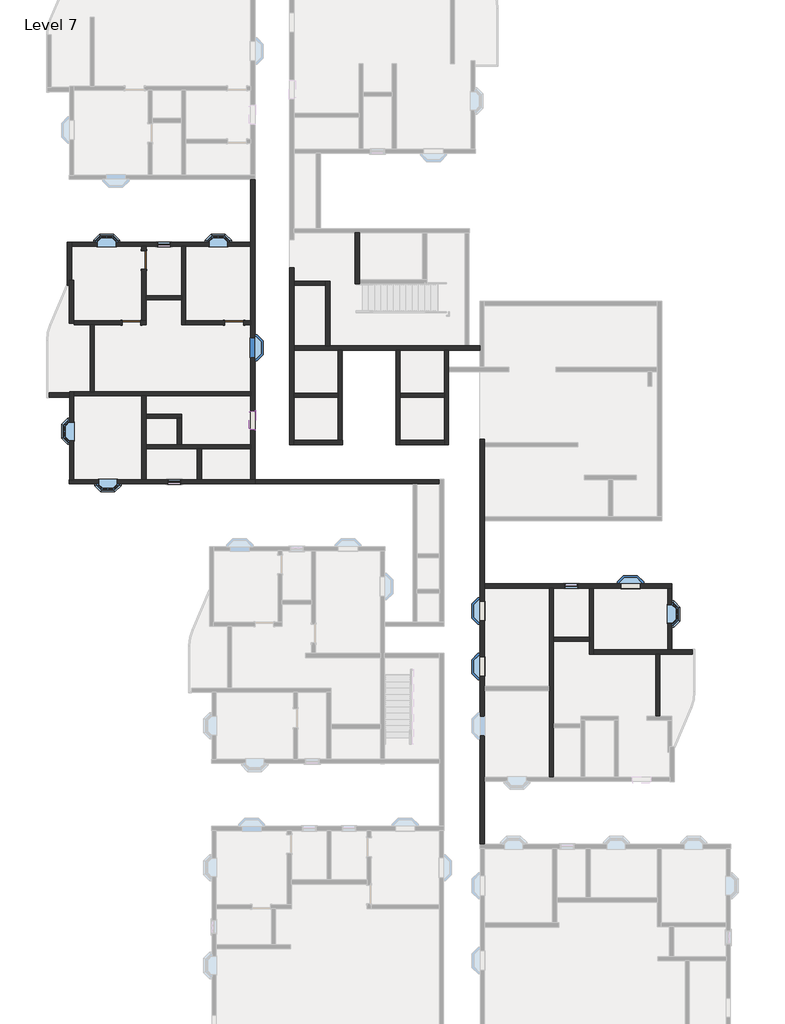
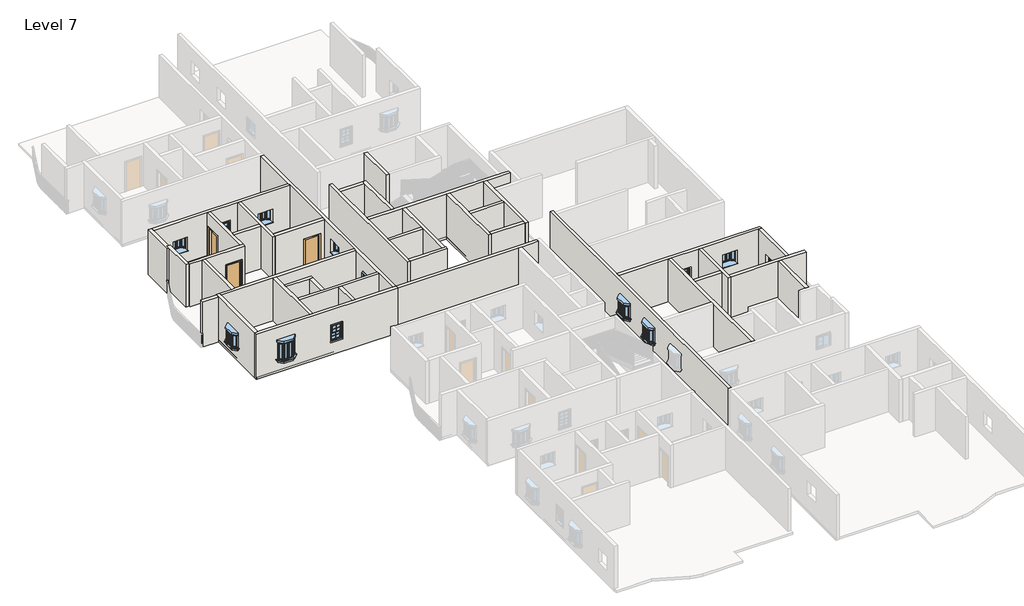
# One storey, part 3 of 14: 40 walls, 13 windows, 3 doors.
"""IFC4 building model written with IfcOpenShell, lengths in millimetres."""

from ifc_helpers import new_model, si_unit, frame, origin, place, context, project, spatial, polyline, outline, extrude, faceted_brep, transform, mapped, element, save
from components import door_54dd4da4, window_910x1210mm_154f9356, window_910x910mm_67ef725a, window_8debb0fa, windows_sgl_w_glazing_bars_910x910mm_256712d0

model = new_model("IFC4")

# Units and contexts
model_context = context("Model", 3, world=origin())
ifc_project = project(units=[si_unit("LENGTHUNIT", "METRE", prefix="MILLI")], contexts=[model_context])

# Site, building, storey
site = spatial("IfcSite", under=ifc_project)
building = spatial("IfcBuilding", under=site)
storey = spatial("IfcBuildingStorey", under=building, Name="Level 7", Elevation=18288.0)

# Doors
placement = place(None, origin())
door_shape = door_54dd4da4(model_context)
element("IfcDoor", 1, ObjectType="Single-Flush : 36\" x 84\"", at=placement, inside=storey, context=model_context, shape_type="MappedRepresentation", body=[
    mapped(door_shape, transform((-11210.3891351, 10605.7083494, 18288.0), x_axis=(1.0, 0.0, 0.0), y_axis=(0.0, 1.0, 0.0), z_axis=(0.0, 0.0, 1.0))),
])
element("IfcDoor", 2, ObjectType="Single-Flush : 36\" x 84\"", at=placement, inside=storey, context=model_context, shape_type="MappedRepresentation", body=[
    mapped(door_shape, transform((-15610.9391351, 13672.7583494, 18288.0), x_axis=(0.0, -1.0, 0.0), y_axis=(1.0, 0.0, 0.0), z_axis=(0.0, 0.0, 1.0))),
])
element("IfcDoor", 3, ObjectType="Single-Flush : 36\" x 84\"", at=placement, inside=storey, context=model_context, shape_type="MappedRepresentation", body=[
    mapped(door_shape, transform((-16220.5391351, 10605.7083494, 18288.0), x_axis=(1.0, 0.0, 0.0), y_axis=(0.0, 1.0, 0.0), z_axis=(0.0, 0.0, 1.0))),
])

# Walls
element("IfcWall", 4, ObjectType="4.5\" p", at=placement, inside=storey, context=model_context, shape_type="Brep", body=[
    faceted_brep([(-15509.3391351, 4456.3873146, 18288.0), (-13007.4391351, 4456.3873146, 18288.0), (-12804.2391351, 4456.3873146, 18288.0), (-10397.5891351, 4456.3873146, 18288.0), (-10397.5891351, 4456.3873146, 21336.0), (-12804.2391351, 4456.3873146, 21336.0), (-13007.4391351, 4456.3873146, 21336.0), (-15509.3391351, 4456.3873146, 21336.0), (-15509.3391351, 4659.5873146, 18288.0), (-15509.3391351, 4659.5873146, 21336.0), (-13985.3391351, 4659.5873146, 21336.0), (-13782.1391351, 4659.5873146, 21336.0), (-10397.5891351, 4659.5873146, 21336.0), (-10397.5891351, 4659.5873146, 18288.0), (-13782.1391351, 4659.5873146, 18288.0), (-13985.3391351, 4659.5873146, 18288.0)], [[[0, 1, 2, 3, 4, 5, 6, 7]], [[8, 9, 10, 11, 12, 13, 14, 15]], [[3, 2, 1, 0, 8, 15, 14, 13]], [[7, 6, 5, 4, 12, 11, 10, 9]], [[4, 3, 13, 12]], [[0, 7, 9, 8]]]),
])
element("IfcWall", 5, ObjectType="4.5\" p", at=placement, inside=storey, context=model_context, shape_type="SweptSolid", body=[
    extrude(outline(polyline([(-13007.4391351, 2953.9583494), (-13007.4391351, 4456.3873146), (-12804.2391351, 4456.3873146), (-12804.2391351, 2953.9583494), (-13007.4391351, 2953.9583494)])), frame((0.0, 0.0, 18288.0), z_axis=(0.0, 0.0, 1.0), x_axis=(1.0, 0.0, 0.0)), (0.0, 0.0, 1.0), 3048.0),
])
element("IfcWall", 6, ObjectType="4.5\" p", at=placement, inside=storey, context=model_context, shape_type="Brep", body=[
    faceted_brep([(-15509.3391351, 5953.2975261, 18288.0), (-13985.3391351, 5953.2975261, 18288.0), (-13782.1391351, 5953.2975261, 18288.0), (-13782.1391351, 5953.2975261, 21336.0), (-13985.3391351, 5953.2975261, 21336.0), (-15509.3391351, 5953.2975261, 21336.0), (-15509.3391351, 6156.4975261, 18288.0), (-15509.3391351, 6156.4975261, 21336.0), (-13782.1391351, 6156.4975261, 21336.0), (-13782.1391351, 6156.4975261, 18288.0)], [[[0, 1, 2, 3, 4, 5]], [[6, 7, 8, 9]], [[2, 1, 0, 6, 9]], [[5, 4, 3, 8, 7]], [[0, 5, 7, 6]], [[3, 2, 9, 8]]]),
])
element("IfcWall", 7, ObjectType="4.5\" p", at=placement, inside=storey, context=model_context, shape_type="SweptSolid", body=[
    extrude(outline(polyline([(-13985.3391351, 4659.5873146), (-13985.3391351, 5953.2975261), (-13782.1391351, 5953.2975261), (-13782.1391351, 4659.5873146), (-13985.3391351, 4659.5873146)])), frame((0.0, 0.0, 18288.0), z_axis=(0.0, 0.0, 1.0), x_axis=(1.0, 0.0, 0.0)), (0.0, 0.0, 1.0), 3048.0),
])
element("IfcWall", 8, ObjectType="4.5\" p", at=placement, inside=storey, context=model_context, shape_type="Brep", body=[
    faceted_brep([(-15712.5391351, 13215.5583494, 20421.6), (-15712.5391351, 13215.5583494, 18288.0), (-15712.5391351, 10707.3083494, 18288.0), (-15712.5391351, 10707.3083494, 21336.0), (-15712.5391351, 14333.1583494, 21336.0), (-15712.5391351, 14333.1583494, 18288.0), (-15712.5391351, 14129.9583494, 18288.0), (-15712.5391351, 14129.9583494, 20421.6), (-15509.3391351, 10707.3083494, 18288.0), (-15509.3391351, 11723.3083494, 18288.0), (-15509.3391351, 11926.5083494, 18288.0), (-15509.3391351, 13215.5583494, 18288.0), (-15509.3391351, 13215.5583494, 20421.6), (-15509.3391351, 14129.9583494, 20421.6), (-15509.3391351, 14129.9583494, 18288.0), (-15509.3391351, 14333.1583494, 18288.0), (-15509.3391351, 14333.1583494, 21336.0), (-15509.3391351, 11926.5083494, 21336.0), (-15509.3391351, 11723.3083494, 21336.0), (-15509.3391351, 10707.3083494, 21336.0)], [[[0, 1, 2, 3, 4, 5, 6, 7]], [[8, 9, 10, 11, 12, 13, 14, 15, 16, 17, 18, 19]], [[6, 5, 15, 14]], [[2, 1, 11, 10, 9, 8]], [[4, 3, 19, 18, 17, 16]], [[3, 2, 8, 19]], [[5, 4, 16, 15]], [[12, 11, 1, 0]], [[13, 12, 0, 7]], [[14, 13, 7, 6]]]),
])
element("IfcWall", 9, ObjectType="4.5\" p", at=placement, inside=storey, context=model_context, shape_type="Brep", body=[
    faceted_brep([(-13769.4391351, 14333.1583494, 18288.0), (-13769.4391351, 11926.5083494, 18288.0), (-13769.4391351, 11723.3083494, 18288.0), (-13769.4391351, 10504.1083494, 18288.0), (-13769.4391351, 10504.1083494, 21336.0), (-13769.4391351, 11723.3083494, 21336.0), (-13769.4391351, 11926.5083494, 21336.0), (-13769.4391351, 14333.1583494, 21336.0), (-13566.2391351, 14333.1583494, 18288.0), (-13566.2391351, 14333.1583494, 21336.0), (-13566.2391351, 10707.3083494, 21336.0), (-13566.2391351, 10504.1083494, 21336.0), (-13566.2391351, 10504.1083494, 18288.0), (-13566.2391351, 10707.3083494, 18288.0)], [[[0, 1, 2, 3, 4, 5, 6, 7]], [[8, 9, 10, 11, 12, 13]], [[3, 2, 1, 0, 8, 13, 12]], [[7, 6, 5, 4, 11, 10, 9]], [[0, 7, 9, 8]], [[4, 3, 12, 11]]]),
])
element("IfcWall", 10, ObjectType="4.5\" p", at=placement, inside=storey, context=model_context, shape_type="SweptSolid", body=[
    extrude(outline(polyline([(20421.6, -10753.1891351), (18288.0, -10753.1891351), (18288.0, -10397.5891351), (21336.0, -10397.5891351), (21336.0, -13566.2391351), (18288.0, -13566.2391351), (18288.0, -11667.5891351), (20421.6, -11667.5891351), (20421.6, -10753.1891351)])), frame((0.0, 10504.1083494, 0.0), z_axis=(0.0, 1.0, 0.0), x_axis=(0.0, 0.0, 1.0)), (0.0, 0.0, 1.0), 203.2),
])
element("IfcWall", 11, ObjectType="4.5\" p", at=placement, inside=storey, context=model_context, shape_type="SweptSolid", body=[
    extrude(outline(polyline([(-13769.4391351, 11723.3083494), (-15509.3391351, 11723.3083494), (-15509.3391351, 11926.5083494), (-13769.4391351, 11926.5083494), (-13769.4391351, 11723.3083494)])), frame((0.0, 0.0, 18288.0), z_axis=(0.0, 0.0, 1.0), x_axis=(1.0, 0.0, 0.0)), (0.0, 0.0, 1.0), 3048.0),
])
element("IfcWall", 12, ObjectType="4.5\" p", at=placement, inside=storey, context=model_context, shape_type="SweptSolid", body=[
    extrude(outline(polyline([(-6739.9891351, 12429.8715905), (-8289.3891351, 12429.8715905), (-8289.3891351, 12633.0715905), (-6739.9891351, 12633.0715905), (-6739.9891351, 12429.8715905)])), frame((0.0, 0.0, 18288.0), z_axis=(0.0, 0.0, 1.0), x_axis=(1.0, 0.0, 0.0)), (0.0, 0.0, 1.0), 3048.0),
])
element("IfcWall", 13, ObjectType="4.5\" p", at=placement, inside=storey, context=model_context, shape_type="SweptSolid", body=[
    extrude(outline(polyline([(-6130.3891351, 6970.2449943), (-8289.3891351, 6970.2449943), (-8289.3891351, 7173.4449943), (-6130.3891351, 7173.4449943), (-6130.3891351, 6970.2449943)])), frame((0.0, 0.0, 18288.0), z_axis=(0.0, 0.0, 1.0), x_axis=(1.0, 0.0, 0.0)), (0.0, 0.0, 1.0), 3048.0),
])
element("IfcWall", 14, ObjectType="4.5\" p", at=placement, inside=storey, context=model_context, shape_type="SweptSolid", body=[
    extrude(outline(polyline([(-948.7891351, 6970.2449943), (-3107.7891351, 6970.2449943), (-3107.7891351, 7173.4449943), (-948.7891351, 7173.4449943), (-948.7891351, 6970.2449943)])), frame((0.0, 0.0, 18288.0), z_axis=(0.0, 0.0, 1.0), x_axis=(1.0, 0.0, 0.0)), (0.0, 0.0, 1.0), 3048.0),
])
element("IfcWall", 15, ObjectType="4.5\" p", at=placement, inside=storey, context=model_context, shape_type="Brep", body=[
    faceted_brep([(-5298.5391351, 14988.9215905, 18288.0), (-5298.5391351, 12506.0715905, 18288.0), (-5298.5391351, 12506.0715905, 21336.0), (-5298.5391351, 14988.9215905, 21336.0), (-5095.3391351, 14988.9215905, 18288.0), (-5095.3391351, 14988.9215905, 21336.0), (-5095.3391351, 12709.2715905, 21336.0), (-5095.3391351, 12506.0715905, 21336.0), (-5095.3391351, 12506.0715905, 18288.0), (-5095.3391351, 12709.2715905, 18288.0)], [[[0, 1, 2, 3]], [[4, 5, 6, 7, 8, 9]], [[1, 0, 4, 9, 8]], [[3, 2, 7, 6, 5]], [[0, 3, 5, 4]], [[2, 1, 8, 7]]]),
])
element("IfcWall", 16, ObjectType="4.5\" p", at=placement, inside=storey, context=model_context, shape_type="SweptSolid", body=[
    extrude(outline(polyline([(-948.7891351, 4665.1949943), (-3107.7891351, 4665.1949943), (-3107.7891351, 4868.3949943), (-948.7891351, 4868.3949943), (-948.7891351, 4665.1949943)])), frame((0.0, 0.0, 18288.0), z_axis=(0.0, 0.0, 1.0), x_axis=(1.0, 0.0, 0.0)), (0.0, 0.0, 1.0), 3048.0),
])
element("IfcWall", 17, ObjectType="4.5\" p", at=placement, inside=storey, context=model_context, shape_type="Brep", body=[
    faceted_brep([(4184.4880523, -2336.4042694, 18288.0), (4184.4880523, -7130.6542694, 18288.0), (4184.4880523, -7333.8542694, 18288.0), (4184.4880523, -11556.6042694, 18288.0), (4184.4880523, -11556.6042694, 21336.0), (4184.4880523, -7333.8542694, 21336.0), (4184.4880523, -7130.6542694, 21336.0), (4184.4880523, -2336.4042694, 21336.0), (4387.6880523, -2336.4042694, 18288.0), (4387.6880523, -2336.4042694, 21336.0), (4387.6880523, -4736.7042694, 21336.0), (4387.6880523, -4939.9042694, 21336.0), (4387.6880523, -8959.4542694, 21336.0), (4387.6880523, -9162.6542694, 21336.0), (4387.6880523, -11556.6042694, 21336.0), (4387.6880523, -11556.6042694, 18288.0), (4387.6880523, -9162.6542694, 18288.0), (4387.6880523, -8959.4542694, 18288.0), (4387.6880523, -4939.9042694, 18288.0), (4387.6880523, -4736.7042694, 18288.0)], [[[0, 1, 2, 3, 4, 5, 6, 7]], [[8, 9, 10, 11, 12, 13, 14, 15, 16, 17, 18, 19]], [[3, 2, 1, 0, 8, 19, 18, 17, 16, 15]], [[7, 6, 5, 4, 14, 13, 12, 11, 10, 9]], [[4, 3, 15, 14]], [[0, 7, 9, 8]]]),
])
element("IfcWall", 18, ObjectType="4.5\" p", at=placement, inside=storey, context=model_context, shape_type="Brep", body=[
    faceted_brep([(803.8108649, 4915.2957306, 18288.0), (803.8108649, -14845.9042694, 18288.0), (803.8108649, -14845.9042694, 21336.0), (803.8108649, 4915.2957306, 21336.0), (803.8108649, -9516.0542694, 20398.0), (803.8108649, -9516.0542694, 19488.0), (803.8108649, -8606.0542694, 19488.0), (803.8108649, -8606.0542694, 20398.0), (803.8108649, -3909.0042694, 20398.0), (803.8108649, -3909.0042694, 19488.0), (803.8108649, -2999.0042694, 19488.0), (803.8108649, -2999.0042694, 20398.0), (803.8108649, -6620.4542694, 20398.0), (803.8108649, -6620.4542694, 19488.0), (803.8108649, -5710.4542694, 19488.0), (803.8108649, -5710.4542694, 20398.0), (1007.0108649, 4915.2957306, 18288.0), (1007.0108649, 4915.2957306, 21336.0), (1007.0108649, 4754.0949943, 21336.0), (1007.0108649, 4550.8949943, 21336.0), (1007.0108649, 1143.3957306, 21336.0), (1007.0108649, 940.1957306, 21336.0), (1007.0108649, -2133.2042694, 21336.0), (1007.0108649, -2336.4042694, 21336.0), (1007.0108649, -7130.6542694, 21336.0), (1007.0108649, -7333.8542694, 21336.0), (1007.0108649, -11556.6042694, 21336.0), (1007.0108649, -11759.8042694, 21336.0), (1007.0108649, -14845.9042694, 21336.0), (1007.0108649, -14845.9042694, 18288.0), (1007.0108649, -11759.8042694, 18288.0), (1007.0108649, -11556.6042694, 18288.0), (1007.0108649, -7333.8542694, 18288.0), (1007.0108649, -7130.6542694, 18288.0), (1007.0108649, -2336.4042694, 18288.0), (1007.0108649, -2133.2042694, 18288.0), (1007.0108649, 940.1957306, 18288.0), (1007.0108649, 1143.3957306, 18288.0), (1007.0108649, 4550.8949943, 18288.0), (1007.0108649, 4754.0949943, 18288.0), (1007.0108649, -9516.0542694, 20398.0), (1007.0108649, -8606.0542694, 20398.0), (1007.0108649, -8606.0542694, 19488.0), (1007.0108649, -9516.0542694, 19488.0), (1007.0108649, -3909.0042694, 20398.0), (1007.0108649, -2999.0042694, 20398.0), (1007.0108649, -2999.0042694, 19488.0), (1007.0108649, -3909.0042694, 19488.0), (1007.0108649, -6620.4542694, 20398.0), (1007.0108649, -5710.4542694, 20398.0), (1007.0108649, -5710.4542694, 19488.0), (1007.0108649, -6620.4542694, 19488.0)], [[[0, 1, 2, 3], [4, 5, 6, 7], [8, 9, 10, 11], [12, 13, 14, 15]], [[16, 17, 18, 19, 20, 21, 22, 23, 24, 25, 26, 27, 28, 29, 30, 31, 32, 33, 34, 35, 36, 37, 38, 39], [40, 41, 42, 43], [44, 45, 46, 47], [48, 49, 50, 51]], [[1, 0, 16, 39, 38, 37, 36, 35, 34, 33, 32, 31, 30, 29]], [[3, 2, 28, 27, 26, 25, 24, 23, 22, 21, 20, 19, 18, 17]], [[0, 3, 17, 16]], [[2, 1, 29, 28]], [[5, 4, 40, 43]], [[6, 5, 43, 42]], [[7, 6, 42, 41]], [[4, 7, 41, 40]], [[9, 8, 44, 47]], [[10, 9, 47, 46]], [[11, 10, 46, 45]], [[8, 11, 45, 44]], [[13, 12, 48, 51]], [[14, 13, 51, 50]], [[15, 14, 50, 49]], [[12, 15, 49, 48]]]),
])
element("IfcWall", 19, ObjectType="4.5\" p", at=placement, inside=storey, context=model_context, shape_type="SweptSolid", body=[
    extrude(outline(polyline([(6127.5880523, -4939.9042694), (4387.6880523, -4939.9042694), (4387.6880523, -4736.7042694), (6127.5880523, -4736.7042694), (6127.5880523, -4939.9042694)])), frame((0.0, 0.0, 18288.0), z_axis=(0.0, 0.0, 1.0), x_axis=(1.0, 0.0, 0.0)), (0.0, 0.0, 1.0), 3048.0),
])
element("IfcWall", 20, ObjectType="4.5\" p", at=placement, inside=storey, context=model_context, shape_type="Brep", body=[
    faceted_brep([(6127.5880523, -2336.4042694, 18288.0), (6127.5880523, -4736.7042694, 18288.0), (6127.5880523, -4939.9042694, 18288.0), (6127.5880523, -5555.8542694, 18288.0), (6127.5880523, -5555.8542694, 21336.0), (6127.5880523, -4939.9042694, 21336.0), (6127.5880523, -4736.7042694, 21336.0), (6127.5880523, -2336.4042694, 21336.0), (6330.7880523, -2336.4042694, 18288.0), (6330.7880523, -2336.4042694, 21336.0), (6330.7880523, -5352.6542694, 21336.0), (6330.7880523, -5555.8542694, 21336.0), (6330.7880523, -5555.8542694, 18288.0), (6330.7880523, -5352.6542694, 18288.0)], [[[0, 1, 2, 3, 4, 5, 6, 7]], [[8, 9, 10, 11, 12, 13]], [[3, 2, 1, 0, 8, 13, 12]], [[7, 6, 5, 4, 11, 10, 9]], [[0, 7, 9, 8]], [[4, 3, 12, 11]]]),
])
element("IfcWall", 21, ObjectType="4.5\" p", at=placement, inside=storey, context=model_context, shape_type="Brep", body=[
    faceted_brep([(6330.7880523, -5555.8542694, 18288.0), (9371.2322031, -5555.8542694, 18288.0), (9574.4322031, -5555.8542694, 18288.0), (11163.1380523, -5555.8542694, 18288.0), (11163.1380523, -5555.8542694, 21336.0), (9574.4322031, -5555.8542694, 21336.0), (9371.2322031, -5555.8542694, 21336.0), (6330.7880523, -5555.8542694, 21336.0), (6330.7880523, -5352.6542694, 18288.0), (6330.7880523, -5352.6542694, 21336.0), (9956.6380523, -5352.6542694, 21336.0), (10159.8380523, -5352.6542694, 21336.0), (11163.1380523, -5352.6542694, 21336.0), (11163.1380523, -5352.6542694, 18288.0), (10159.8380523, -5352.6542694, 18288.0), (9956.6380523, -5352.6542694, 18288.0)], [[[0, 1, 2, 3, 4, 5, 6, 7]], [[8, 9, 10, 11, 12, 13, 14, 15]], [[3, 2, 1, 0, 8, 15, 14, 13]], [[4, 3, 13, 12]], [[7, 6, 5, 4, 12, 11, 10, 9]], [[0, 7, 9, 8]]]),
])
element("IfcWall", 22, ObjectType="4.5\" p", at=placement, inside=storey, context=model_context, shape_type="SweptSolid", body=[
    extrude(outline(polyline([(9371.2322031, -8578.4542694), (9371.2322031, -5555.8542694), (9574.4322031, -5555.8542694), (9574.4322031, -8578.4542694), (9371.2322031, -8578.4542694)])), frame((0.0, 0.0, 18288.0), z_axis=(0.0, 0.0, 1.0), x_axis=(1.0, 0.0, 0.0)), (0.0, 0.0, 1.0), 3048.0),
])
element("IfcWall", 23, ObjectType="9\"", at=placement, inside=storey, context=model_context, shape_type="Brep", body=[
    faceted_brep([(-10181.6891351, 2953.9583494, 18288.0), (-10194.3891351, 2953.9583494, 18288.0), (-10397.5891351, 2953.9583494, 18288.0), (-12804.2391351, 2953.9583494, 18288.0), (-13007.4391351, 2953.9583494, 18288.0), (-15509.3391351, 2953.9583494, 18288.0), (-15712.5391351, 2953.9583494, 18288.0), (-19033.5891351, 2953.9583494, 18288.0), (-19236.7891351, 2953.9583494, 18288.0), (-19249.4891351, 2953.9583494, 18288.0), (-19249.4891351, 2953.9583494, 21336.0), (-19236.7891351, 2953.9583494, 21336.0), (-19033.5891351, 2953.9583494, 21336.0), (-15712.5391351, 2953.9583494, 21336.0), (-15509.3391351, 2953.9583494, 21336.0), (-13007.4391351, 2953.9583494, 21336.0), (-12804.2391351, 2953.9583494, 21336.0), (-10397.5891351, 2953.9583494, 21336.0), (-10194.3891351, 2953.9583494, 21336.0), (-10181.6891351, 2953.9583494, 21336.0), (-13794.8391351, 2953.9583494, 20269.2), (-14455.2391351, 2953.9583494, 20269.2), (-14455.2391351, 2953.9583494, 19202.4), (-13794.8391351, 2953.9583494, 19202.4), (-16918.0641351, 2953.9583494, 20398.0), (-17828.0641351, 2953.9583494, 20398.0), (-17828.0641351, 2953.9583494, 19188.0), (-16918.0641351, 2953.9583494, 19188.0), (-10181.6891351, 2750.7583494, 18288.0), (-10181.6891351, 2750.7583494, 21336.0), (-19249.4891351, 2750.7583494, 21336.0), (-19249.4891351, 2750.7583494, 18288.0), (-13794.8391351, 2750.7583494, 20269.2), (-13794.8391351, 2750.7583494, 19202.4), (-14455.2391351, 2750.7583494, 19202.4), (-14455.2391351, 2750.7583494, 20269.2), (-16918.0641351, 2750.7583494, 20398.0), (-16918.0641351, 2750.7583494, 19188.0), (-17828.0641351, 2750.7583494, 19188.0), (-17828.0641351, 2750.7583494, 20398.0)], [[[0, 1, 2, 3, 4, 5, 6, 7, 8, 9, 10, 11, 12, 13, 14, 15, 16, 17, 18, 19], [20, 21, 22, 23], [24, 25, 26, 27]], [[28, 29, 30, 31], [32, 33, 34, 35], [36, 37, 38, 39]], [[9, 8, 7, 6, 5, 4, 3, 2, 1, 0, 28, 31]], [[10, 9, 31, 30]], [[19, 18, 17, 16, 15, 14, 13, 12, 11, 10, 30, 29]], [[0, 19, 29, 28]], [[33, 32, 20, 23]], [[34, 33, 23, 22]], [[35, 34, 22, 21]], [[32, 35, 21, 20]], [[37, 36, 24, 27]], [[38, 37, 27, 26]], [[39, 38, 26, 25]], [[36, 39, 25, 24]]]),
])
element("IfcWall", 24, ObjectType="9\"", at=placement, inside=storey, context=model_context, shape_type="Brep", body=[
    faceted_brep([(-19033.5891351, 2953.9583494, 18288.0), (-19033.5891351, 7037.0083494, 18288.0), (-19033.5891351, 7240.2083494, 18288.0), (-19033.5891351, 7240.2083494, 21336.0), (-19033.5891351, 7037.0083494, 21336.0), (-19033.5891351, 2953.9583494, 21336.0), (-19033.5891351, 4854.8083494, 20112.4), (-19033.5891351, 5764.8083494, 20112.4), (-19033.5891351, 5764.8083494, 19202.4), (-19033.5891351, 4854.8083494, 19202.4), (-19236.7891351, 2953.9583494, 18288.0), (-19236.7891351, 2953.9583494, 21336.0), (-19236.7891351, 7240.2083494, 21336.0), (-19236.7891351, 7240.2083494, 18288.0), (-19236.7891351, 4854.8083494, 20112.4), (-19236.7891351, 4854.8083494, 19202.4), (-19236.7891351, 5764.8083494, 19202.4), (-19236.7891351, 5764.8083494, 20112.4)], [[[0, 1, 2, 3, 4, 5], [6, 7, 8, 9]], [[10, 11, 12, 13], [14, 15, 16, 17]], [[2, 1, 0, 10, 13]], [[5, 4, 3, 12, 11]], [[0, 5, 11, 10]], [[3, 2, 13, 12]], [[15, 14, 6, 9]], [[16, 15, 9, 8]], [[17, 16, 8, 7]], [[14, 17, 7, 6]]]),
])
element("IfcWall", 25, ObjectType="9\"", at=placement, inside=storey, context=model_context, shape_type="Brep", body=[
    faceted_brep([(-10194.3891351, 2953.9583494, 18288.0), (-10194.3891351, 17597.0583494, 18288.0), (-10194.3891351, 17597.0583494, 21336.0), (-10194.3891351, 2953.9583494, 21336.0), (-10194.3891351, 9841.5083494, 20398.0), (-10194.3891351, 9841.5083494, 19488.0), (-10194.3891351, 8931.5083494, 19488.0), (-10194.3891351, 8931.5083494, 20398.0), (-10194.3891351, 5393.297832, 20398.0), (-10194.3891351, 6303.297832, 20398.0), (-10194.3891351, 6303.297832, 19488.0), (-10194.3891351, 5393.297832, 19488.0), (-10397.5891351, 2953.9583494, 18288.0), (-10397.5891351, 2953.9583494, 21336.0), (-10397.5891351, 4456.3873146, 21336.0), (-10397.5891351, 4659.5873146, 21336.0), (-10397.5891351, 7037.0083494, 21336.0), (-10397.5891351, 7240.2083494, 21336.0), (-10397.5891351, 10504.1083494, 21336.0), (-10397.5891351, 10707.3083494, 21336.0), (-10397.5891351, 14333.1583494, 21336.0), (-10397.5891351, 14536.3583494, 21336.0), (-10397.5891351, 17597.0583494, 21336.0), (-10397.5891351, 17597.0583494, 18288.0), (-10397.5891351, 14536.3583494, 18288.0), (-10397.5891351, 14333.1583494, 18288.0), (-10397.5891351, 10707.3083494, 18288.0), (-10397.5891351, 10504.1083494, 18288.0), (-10397.5891351, 7240.2083494, 18288.0), (-10397.5891351, 7037.0083494, 18288.0), (-10397.5891351, 4659.5873146, 18288.0), (-10397.5891351, 4456.3873146, 18288.0), (-10397.5891351, 9841.5083494, 20398.0), (-10397.5891351, 8931.5083494, 20398.0), (-10397.5891351, 8931.5083494, 19488.0), (-10397.5891351, 9841.5083494, 19488.0), (-10397.5891351, 5393.297832, 20398.0), (-10397.5891351, 5393.297832, 19488.0), (-10397.5891351, 6303.297832, 19488.0), (-10397.5891351, 6303.297832, 20398.0)], [[[0, 1, 2, 3], [4, 5, 6, 7], [8, 9, 10, 11]], [[12, 13, 14, 15, 16, 17, 18, 19, 20, 21, 22, 23, 24, 25, 26, 27, 28, 29, 30, 31], [32, 33, 34, 35], [36, 37, 38, 39]], [[1, 0, 12, 31, 30, 29, 28, 27, 26, 25, 24, 23]], [[2, 1, 23, 22]], [[3, 2, 22, 21, 20, 19, 18, 17, 16, 15, 14, 13]], [[0, 3, 13, 12]], [[5, 4, 32, 35]], [[6, 5, 35, 34]], [[7, 6, 34, 33]], [[4, 7, 33, 32]], [[37, 36, 8, 11]], [[38, 37, 11, 10]], [[39, 38, 10, 9]], [[36, 39, 9, 8]]]),
])
element("IfcWall", 26, ObjectType="9\"", at=placement, inside=storey, context=model_context, shape_type="SweptSolid", body=[
    extrude(outline(polyline([(-19249.4891351, 6979.8583494), (-20240.0891351, 6979.8583494), (-20240.0891351, 7183.0583494), (-19249.4891351, 7183.0583494), (-19249.4891351, 6979.8583494)])), frame((0.0, 0.0, 18288.0), z_axis=(0.0, 0.0, 1.0), x_axis=(1.0, 0.0, 0.0)), (0.0, 0.0, 1.0), 3048.0),
])
element("IfcWall", 27, ObjectType="9\"", at=placement, inside=storey, context=model_context, shape_type="Brep", body=[
    faceted_brep([(-19147.8891351, 12435.1858981, 18288.0), (-19147.8891351, 14333.1583494, 18288.0), (-19147.8891351, 14536.3583494, 18288.0), (-19147.8891351, 14549.0583494, 18288.0), (-19147.8891351, 14549.0583494, 21336.0), (-19147.8891351, 14536.3583494, 21336.0), (-19147.8891351, 14333.1583494, 21336.0), (-19147.8891351, 12435.1858981, 21336.0), (-19351.0891351, 12435.1858981, 18288.0), (-19351.0891351, 12435.1858981, 21336.0), (-19351.0891351, 14549.0583494, 21336.0), (-19351.0891351, 14549.0583494, 18288.0)], [[[0, 1, 2, 3, 4, 5, 6, 7]], [[8, 9, 10, 11]], [[3, 2, 1, 0, 8, 11]], [[4, 3, 11, 10]], [[7, 6, 5, 4, 10, 9]], [[0, 7, 9, 8]]]),
])
element("IfcWall", 28, ObjectType="9\"", at=placement, inside=storey, context=model_context, shape_type="Brep", body=[
    faceted_brep([(-19147.8891351, 14333.1583494, 18288.0), (-15712.5391351, 14333.1583494, 18288.0), (-15509.3391351, 14333.1583494, 18288.0), (-13769.4391351, 14333.1583494, 18288.0), (-13566.2391351, 14333.1583494, 18288.0), (-10397.5891351, 14333.1583494, 18288.0), (-10397.5891351, 14333.1583494, 21336.0), (-13566.2391351, 14333.1583494, 21336.0), (-13769.4391351, 14333.1583494, 21336.0), (-15509.3391351, 14333.1583494, 21336.0), (-15712.5391351, 14333.1583494, 21336.0), (-19147.8891351, 14333.1583494, 21336.0), (-17885.2141351, 14333.1583494, 20112.4), (-16975.2141351, 14333.1583494, 20112.4), (-16975.2141351, 14333.1583494, 19202.4), (-17885.2141351, 14333.1583494, 19202.4), (-12436.9141351, 14333.1583494, 20112.4), (-11526.9141351, 14333.1583494, 20112.4), (-11526.9141351, 14333.1583494, 19202.4), (-12436.9141351, 14333.1583494, 19202.4), (-14309.1891351, 14333.1583494, 20269.2), (-14309.1891351, 14333.1583494, 19202.4), (-14969.5891351, 14333.1583494, 19202.4), (-14969.5891351, 14333.1583494, 20269.2), (-19147.8891351, 14536.3583494, 18288.0), (-19147.8891351, 14536.3583494, 21336.0), (-10397.5891351, 14536.3583494, 21336.0), (-10397.5891351, 14536.3583494, 18288.0), (-17885.2141351, 14536.3583494, 20112.4), (-17885.2141351, 14536.3583494, 19202.4), (-16975.2141351, 14536.3583494, 19202.4), (-16975.2141351, 14536.3583494, 20112.4), (-12436.9141351, 14536.3583494, 20112.4), (-12436.9141351, 14536.3583494, 19202.4), (-11526.9141351, 14536.3583494, 19202.4), (-11526.9141351, 14536.3583494, 20112.4), (-14309.1891351, 14536.3583494, 20269.2), (-14969.5891351, 14536.3583494, 20269.2), (-14969.5891351, 14536.3583494, 19202.4), (-14309.1891351, 14536.3583494, 19202.4)], [[[0, 1, 2, 3, 4, 5, 6, 7, 8, 9, 10, 11], [12, 13, 14, 15], [16, 17, 18, 19], [20, 21, 22, 23]], [[24, 25, 26, 27], [28, 29, 30, 31], [32, 33, 34, 35], [36, 37, 38, 39]], [[5, 4, 3, 2, 1, 0, 24, 27]], [[11, 10, 9, 8, 7, 6, 26, 25]], [[6, 5, 27, 26]], [[0, 11, 25, 24]], [[29, 28, 12, 15]], [[30, 29, 15, 14]], [[31, 30, 14, 13]], [[28, 31, 13, 12]], [[33, 32, 16, 19]], [[34, 33, 19, 18]], [[35, 34, 18, 17]], [[32, 35, 17, 16]], [[21, 20, 36, 39]], [[22, 21, 39, 38]], [[23, 22, 38, 37]], [[20, 23, 37, 36]]]),
])
element("IfcWall", 29, ObjectType="9\"", at=placement, inside=storey, context=model_context, shape_type="SweptSolid", body=[
    extrude(outline(polyline([(-19249.4891351, 10585.5474528), (-19249.4891351, 12672.4473407), (-19046.2891351, 12672.4473407), (-19046.2891351, 10585.5474528), (-19249.4891351, 10585.5474528)])), frame((0.0, 0.0, 18288.0), z_axis=(0.0, 0.0, 1.0), x_axis=(1.0, 0.0, 0.0)), (0.0, 0.0, 1.0), 3048.0),
])
element("IfcWall", 30, ObjectType="9\" w", at=placement, inside=storey, context=model_context, shape_type="Brep", body=[
    faceted_brep([(-1177.3891351, 2953.9583494, 18288.0), (-10181.6891351, 2953.9583494, 18288.0), (-10181.6891351, 2953.9583494, 21336.0), (-1177.3891351, 2953.9583494, 21336.0), (-1177.3891351, 2750.7583494, 18288.0), (-1177.3891351, 2750.7583494, 21336.0), (-2269.5891351, 2750.7583494, 21336.0), (-2472.7891351, 2750.7583494, 21336.0), (-10181.6891351, 2750.7583494, 21336.0), (-10181.6891351, 2750.7583494, 18288.0), (-2472.7891351, 2750.7583494, 18288.0), (-2269.5891351, 2750.7583494, 18288.0)], [[[0, 1, 2, 3]], [[4, 5, 6, 7, 8, 9, 10, 11]], [[1, 0, 4, 11, 10, 9]], [[2, 1, 9, 8]], [[3, 2, 8, 7, 6, 5]], [[0, 3, 5, 4]]]),
])
element("IfcWall", 31, ObjectType="9\" w", at=placement, inside=storey, context=model_context, shape_type="Brep", body=[
    faceted_brep([(-15763.3391351, 10504.1083494, 20421.6), (-15763.3391351, 10504.1083494, 18288.0), (-15509.3391351, 10504.1083494, 18288.0), (-15509.3391351, 10504.1083494, 21336.0), (-18042.9891351, 10504.1083494, 21336.0), (-18246.1891351, 10504.1083494, 21336.0), (-19027.2391351, 10504.1083494, 21336.0), (-19027.2391351, 10504.1083494, 18288.0), (-18246.1891351, 10504.1083494, 18288.0), (-18042.9891351, 10504.1083494, 18288.0), (-16677.7391351, 10504.1083494, 18288.0), (-16677.7391351, 10504.1083494, 20421.6), (-15509.3391351, 10707.3083494, 18288.0), (-15712.5391351, 10707.3083494, 18288.0), (-15763.3391351, 10707.3083494, 18288.0), (-15763.3391351, 10707.3083494, 20421.6), (-16677.7391351, 10707.3083494, 20421.6), (-16677.7391351, 10707.3083494, 18288.0), (-19027.2391351, 10707.3083494, 18288.0), (-19027.2391351, 10707.3083494, 21336.0), (-15712.5391351, 10707.3083494, 21336.0), (-15509.3391351, 10707.3083494, 21336.0)], [[[0, 1, 2, 3, 4, 5, 6, 7, 8, 9, 10, 11]], [[12, 13, 14, 15, 16, 17, 18, 19, 20, 21]], [[2, 1, 14, 13, 12]], [[10, 9, 8, 7, 18, 17]], [[6, 5, 4, 3, 21, 20, 19]], [[7, 6, 19, 18]], [[3, 2, 12, 21]], [[15, 14, 1, 0]], [[16, 15, 0, 11]], [[17, 16, 11, 10]]]),
])
element("IfcWall", 32, ObjectType="9\" w", at=placement, inside=storey, context=model_context, shape_type="SweptSolid", body=[
    extrude(outline(polyline([(-18246.1891351, 7240.2083494), (-18246.1891351, 10504.1083494), (-18042.9891351, 10504.1083494), (-18042.9891351, 7240.2083494), (-18246.1891351, 7240.2083494)])), frame((0.0, 0.0, 18288.0), z_axis=(0.0, 0.0, 1.0), x_axis=(1.0, 0.0, 0.0)), (0.0, 0.0, 1.0), 3048.0),
])
element("IfcWall", 33, ObjectType="9\" w", at=placement, inside=storey, context=model_context, shape_type="Brep", body=[
    faceted_brep([(-19033.5891351, 7037.0083494, 18288.0), (-15712.5391351, 7037.0083494, 18288.0), (-15509.3391351, 7037.0083494, 18288.0), (-10397.5891351, 7037.0083494, 18288.0), (-10397.5891351, 7037.0083494, 21336.0), (-15509.3391351, 7037.0083494, 21336.0), (-15712.5391351, 7037.0083494, 21336.0), (-19033.5891351, 7037.0083494, 21336.0), (-19033.5891351, 7240.2083494, 18288.0), (-19033.5891351, 7240.2083494, 21336.0), (-18246.1891351, 7240.2083494, 21336.0), (-18042.9891351, 7240.2083494, 21336.0), (-10397.5891351, 7240.2083494, 21336.0), (-10397.5891351, 7240.2083494, 18288.0), (-18042.9891351, 7240.2083494, 18288.0), (-18246.1891351, 7240.2083494, 18288.0)], [[[0, 1, 2, 3, 4, 5, 6, 7]], [[8, 9, 10, 11, 12, 13, 14, 15]], [[3, 2, 1, 0, 8, 15, 14, 13]], [[7, 6, 5, 4, 12, 11, 10, 9]], [[0, 7, 9, 8]], [[4, 3, 13, 12]]]),
])
element("IfcWall", 34, ObjectType="9\" w", at=placement, inside=storey, context=model_context, shape_type="Brep", body=[
    faceted_brep([(-15712.5391351, 7037.0083494, 18288.0), (-15712.5391351, 2953.9583494, 18288.0), (-15712.5391351, 2953.9583494, 21336.0), (-15712.5391351, 7037.0083494, 21336.0), (-15509.3391351, 7037.0083494, 18288.0), (-15509.3391351, 7037.0083494, 21336.0), (-15509.3391351, 6156.4975261, 21336.0), (-15509.3391351, 5953.2975261, 21336.0), (-15509.3391351, 4659.5873146, 21336.0), (-15509.3391351, 4456.3873146, 21336.0), (-15509.3391351, 2953.9583494, 21336.0), (-15509.3391351, 2953.9583494, 18288.0), (-15509.3391351, 4456.3873146, 18288.0), (-15509.3391351, 4659.5873146, 18288.0), (-15509.3391351, 5953.2975261, 18288.0), (-15509.3391351, 6156.4975261, 18288.0)], [[[0, 1, 2, 3]], [[4, 5, 6, 7, 8, 9, 10, 11, 12, 13, 14, 15]], [[1, 0, 4, 15, 14, 13, 12, 11]], [[3, 2, 10, 9, 8, 7, 6, 5]], [[2, 1, 11, 10]], [[0, 3, 5, 4]]]),
])
element("IfcWall", 35, ObjectType="9\" w", at=placement, inside=storey, context=model_context, shape_type="Brep", body=[
    faceted_brep([(-8492.5891351, 13295.1410318, 18288.0), (-8492.5891351, 4652.4949943, 18288.0), (-8492.5891351, 4652.4949943, 21336.0), (-8492.5891351, 13295.1410318, 21336.0), (-8289.3891351, 13295.1410318, 18288.0), (-8289.3891351, 13295.1410318, 21336.0), (-8289.3891351, 12633.0715905, 21336.0), (-8289.3891351, 12429.8715905, 21336.0), (-8289.3891351, 9478.4949943, 21336.0), (-8289.3891351, 9275.2949943, 21336.0), (-8289.3891351, 7173.4449943, 21336.0), (-8289.3891351, 6970.2449943, 21336.0), (-8289.3891351, 4868.3949943, 21336.0), (-8289.3891351, 4665.1949943, 21336.0), (-8289.3891351, 4652.4949943, 21336.0), (-8289.3891351, 4652.4949943, 18288.0), (-8289.3891351, 4665.1949943, 18288.0), (-8289.3891351, 4868.3949943, 18288.0), (-8289.3891351, 6970.2449943, 18288.0), (-8289.3891351, 7173.4449943, 18288.0), (-8289.3891351, 9275.2949943, 18288.0), (-8289.3891351, 9478.4949943, 18288.0), (-8289.3891351, 12429.8715905, 18288.0), (-8289.3891351, 12633.0715905, 18288.0)], [[[0, 1, 2, 3]], [[4, 5, 6, 7, 8, 9, 10, 11, 12, 13, 14, 15, 16, 17, 18, 19, 20, 21, 22, 23]], [[1, 0, 4, 23, 22, 21, 20, 19, 18, 17, 16, 15]], [[2, 1, 15, 14]], [[3, 2, 14, 13, 12, 11, 10, 9, 8, 7, 6, 5]], [[0, 3, 5, 4]]]),
])
element("IfcWall", 36, ObjectType="9\" w", at=placement, inside=storey, context=model_context, shape_type="Brep", body=[
    faceted_brep([(-8289.3891351, 4665.1949943, 18288.0), (-5914.4891351, 4665.1949943, 18288.0), (-5914.4891351, 4665.1949943, 21336.0), (-8289.3891351, 4665.1949943, 21336.0), (-8289.3891351, 4868.3949943, 18288.0), (-8289.3891351, 4868.3949943, 21336.0), (-6130.3891351, 4868.3949943, 21336.0), (-5927.1891351, 4868.3949943, 21336.0), (-5914.4891351, 4868.3949943, 21336.0), (-5914.4891351, 4868.3949943, 18288.0), (-5927.1891351, 4868.3949943, 18288.0), (-6130.3891351, 4868.3949943, 18288.0)], [[[0, 1, 2, 3]], [[4, 5, 6, 7, 8, 9, 10, 11]], [[1, 0, 4, 11, 10, 9]], [[2, 1, 9, 8]], [[3, 2, 8, 7, 6, 5]], [[0, 3, 5, 4]]]),
])
element("IfcWall", 37, ObjectType="9\" w", at=placement, inside=storey, context=model_context, shape_type="Brep", body=[
    faceted_brep([(-5927.1891351, 4868.3949943, 18288.0), (-5927.1891351, 9275.2949943, 18288.0), (-5927.1891351, 9275.2949943, 21336.0), (-5927.1891351, 4868.3949943, 21336.0), (-6130.3891351, 4868.3949943, 18288.0), (-6130.3891351, 4868.3949943, 21336.0), (-6130.3891351, 6970.2449943, 21336.0), (-6130.3891351, 7173.4449943, 21336.0), (-6130.3891351, 9275.2949943, 21336.0), (-6130.3891351, 9275.2949943, 18288.0), (-6130.3891351, 7173.4449943, 18288.0), (-6130.3891351, 6970.2449943, 18288.0)], [[[0, 1, 2, 3]], [[4, 5, 6, 7, 8, 9, 10, 11]], [[1, 0, 4, 11, 10, 9]], [[3, 2, 8, 7, 6, 5]], [[0, 3, 5, 4]], [[2, 1, 9, 8]]]),
])
element("IfcWall", 38, ObjectType="9\" w", at=placement, inside=storey, context=model_context, shape_type="Brep", body=[
    faceted_brep([(-8289.3891351, 9275.2949943, 18288.0), (-6130.3891351, 9275.2949943, 18288.0), (-5927.1891351, 9275.2949943, 18288.0), (-3310.9891351, 9275.2949943, 18288.0), (-3107.7891351, 9275.2949943, 18288.0), (-948.7891351, 9275.2949943, 18288.0), (-745.5891351, 9275.2949943, 18288.0), (793.5880523, 9275.2949943, 18288.0), (793.5880523, 9275.2949943, 21336.0), (-745.5891351, 9275.2949943, 21336.0), (-948.7891351, 9275.2949943, 21336.0), (-3107.7891351, 9275.2949943, 21336.0), (-3310.9891351, 9275.2949943, 21336.0), (-5927.1891351, 9275.2949943, 21336.0), (-6130.3891351, 9275.2949943, 21336.0), (-8289.3891351, 9275.2949943, 21336.0), (-8289.3891351, 9478.4949943, 18288.0), (-8289.3891351, 9478.4949943, 21336.0), (-6739.9891351, 9478.4949943, 21336.0), (-6536.7891351, 9478.4949943, 21336.0), (54.5108649, 9478.4949943, 21336.0), (257.7108649, 9478.4949943, 21336.0), (793.5880523, 9478.4949943, 21336.0), (793.5880523, 9478.4949943, 18288.0), (257.7108649, 9478.4949943, 18288.0), (54.5108649, 9478.4949943, 18288.0), (-6536.7891351, 9478.4949943, 18288.0), (-6739.9891351, 9478.4949943, 18288.0)], [[[0, 1, 2, 3, 4, 5, 6, 7, 8, 9, 10, 11, 12, 13, 14, 15]], [[16, 17, 18, 19, 20, 21, 22, 23, 24, 25, 26, 27]], [[7, 6, 5, 4, 3, 2, 1, 0, 16, 27, 26, 25, 24, 23]], [[15, 14, 13, 12, 11, 10, 9, 8, 22, 21, 20, 19, 18, 17]], [[0, 15, 17, 16]], [[8, 7, 23, 22]]]),
])
element("IfcWall", 39, ObjectType="9\" w", at=placement, inside=storey, context=model_context, shape_type="Brep", body=[
    faceted_brep([(-3310.9891351, 9275.2949943, 18288.0), (-3310.9891351, 4652.4949943, 18288.0), (-3310.9891351, 4652.4949943, 21336.0), (-3310.9891351, 9275.2949943, 21336.0), (-3107.7891351, 9275.2949943, 18288.0), (-3107.7891351, 9275.2949943, 21336.0), (-3107.7891351, 7173.4449943, 21336.0), (-3107.7891351, 6970.2449943, 21336.0), (-3107.7891351, 4868.3949943, 21336.0), (-3107.7891351, 4665.1949943, 21336.0), (-3107.7891351, 4652.4949943, 21336.0), (-3107.7891351, 4652.4949943, 18288.0), (-3107.7891351, 4665.1949943, 18288.0), (-3107.7891351, 4868.3949943, 18288.0), (-3107.7891351, 6970.2449943, 18288.0), (-3107.7891351, 7173.4449943, 18288.0)], [[[0, 1, 2, 3]], [[4, 5, 6, 7, 8, 9, 10, 11, 12, 13, 14, 15]], [[1, 0, 4, 15, 14, 13, 12, 11]], [[2, 1, 11, 10]], [[3, 2, 10, 9, 8, 7, 6, 5]], [[0, 3, 5, 4]]]),
])
element("IfcWall", 40, ObjectType="9\" w", at=placement, inside=storey, context=model_context, shape_type="Brep", body=[
    faceted_brep([(-745.5891351, 4652.4949943, 18288.0), (-745.5891351, 8223.6457306, 18288.0), (-745.5891351, 8426.8457306, 18288.0), (-745.5891351, 9275.2949943, 18288.0), (-745.5891351, 9275.2949943, 21336.0), (-745.5891351, 8426.8457306, 21336.0), (-745.5891351, 8223.6457306, 21336.0), (-745.5891351, 4652.4949943, 21336.0), (-948.7891351, 4652.4949943, 18288.0), (-948.7891351, 4652.4949943, 21336.0), (-948.7891351, 4665.1949943, 21336.0), (-948.7891351, 4868.3949943, 21336.0), (-948.7891351, 6970.2449943, 21336.0), (-948.7891351, 7173.4449943, 21336.0), (-948.7891351, 9275.2949943, 21336.0), (-948.7891351, 9275.2949943, 18288.0), (-948.7891351, 7173.4449943, 18288.0), (-948.7891351, 6970.2449943, 18288.0), (-948.7891351, 4868.3949943, 18288.0), (-948.7891351, 4665.1949943, 18288.0)], [[[0, 1, 2, 3, 4, 5, 6, 7]], [[8, 9, 10, 11, 12, 13, 14, 15, 16, 17, 18, 19]], [[3, 2, 1, 0, 8, 19, 18, 17, 16, 15]], [[7, 6, 5, 4, 14, 13, 12, 11, 10, 9]], [[0, 7, 9, 8]], [[4, 3, 15, 14]]]),
])
element("IfcWall", 41, ObjectType="9\" w", at=placement, inside=storey, context=model_context, shape_type="Brep", body=[
    faceted_brep([(-6536.7891351, 9478.4949943, 18288.0), (-6536.7891351, 12633.0715905, 18288.0), (-6536.7891351, 12633.0715905, 21336.0), (-6536.7891351, 9478.4949943, 21336.0), (-6739.9891351, 9478.4949943, 18288.0), (-6739.9891351, 9478.4949943, 21336.0), (-6739.9891351, 12429.8715905, 21336.0), (-6739.9891351, 12633.0715905, 21336.0), (-6739.9891351, 12633.0715905, 18288.0), (-6739.9891351, 12429.8715905, 18288.0)], [[[0, 1, 2, 3]], [[4, 5, 6, 7, 8, 9]], [[1, 0, 4, 9, 8]], [[3, 2, 7, 6, 5]], [[0, 3, 5, 4]], [[2, 1, 8, 7]]]),
])
element("IfcWall", 42, ObjectType="9\" w", at=placement, inside=storey, context=model_context, shape_type="Brep", body=[
    faceted_brep([(1007.0108649, -2336.4042694, 18288.0), (4184.4880523, -2336.4042694, 18288.0), (4387.6880523, -2336.4042694, 18288.0), (6127.5880523, -2336.4042694, 18288.0), (6330.7880523, -2336.4042694, 18288.0), (9956.6380523, -2336.4042694, 18288.0), (10159.8380523, -2336.4042694, 18288.0), (10172.5380523, -2336.4042694, 18288.0), (10172.5380523, -2336.4042694, 21336.0), (10159.8380523, -2336.4042694, 21336.0), (9956.6380523, -2336.4042694, 21336.0), (6330.7880523, -2336.4042694, 21336.0), (6127.5880523, -2336.4042694, 21336.0), (4387.6880523, -2336.4042694, 21336.0), (4184.4880523, -2336.4042694, 21336.0), (1007.0108649, -2336.4042694, 21336.0), (7688.7130523, -2336.4042694, 20398.0), (8598.7130523, -2336.4042694, 20398.0), (8598.7130523, -2336.4042694, 19488.0), (7688.7130523, -2336.4042694, 19488.0), (4927.4380523, -2336.4042694, 20269.2), (5587.8380523, -2336.4042694, 20269.2), (5587.8380523, -2336.4042694, 19202.4), (4927.4380523, -2336.4042694, 19202.4), (1007.0108649, -2133.2042694, 18288.0), (1007.0108649, -2133.2042694, 21336.0), (10172.5380523, -2133.2042694, 21336.0), (10172.5380523, -2133.2042694, 18288.0), (7688.7130523, -2133.2042694, 20398.0), (7688.7130523, -2133.2042694, 19488.0), (8598.7130523, -2133.2042694, 19488.0), (8598.7130523, -2133.2042694, 20398.0), (4927.4380523, -2133.2042694, 20269.2), (4927.4380523, -2133.2042694, 19202.4), (5587.8380523, -2133.2042694, 19202.4), (5587.8380523, -2133.2042694, 20269.2)], [[[0, 1, 2, 3, 4, 5, 6, 7, 8, 9, 10, 11, 12, 13, 14, 15], [16, 17, 18, 19], [20, 21, 22, 23]], [[24, 25, 26, 27], [28, 29, 30, 31], [32, 33, 34, 35]], [[7, 6, 5, 4, 3, 2, 1, 0, 24, 27]], [[8, 7, 27, 26]], [[15, 14, 13, 12, 11, 10, 9, 8, 26, 25]], [[0, 15, 25, 24]], [[29, 28, 16, 19]], [[30, 29, 19, 18]], [[31, 30, 18, 17]], [[28, 31, 17, 16]], [[33, 32, 20, 23]], [[34, 33, 23, 22]], [[35, 34, 22, 21]], [[32, 35, 21, 20]]]),
])
element("IfcWall", 43, ObjectType="9\" w", at=placement, inside=storey, context=model_context, shape_type="SweptSolid", body=[
    extrude(outline(polyline([(-2336.4042694, 18288.0), (-5352.6542694, 18288.0), (-5352.6542694, 21336.0), (-2336.4042694, 21336.0), (-2336.4042694, 18288.0)]), holes=[polyline([(-3151.4042694, 20112.4), (-4061.4042694, 20112.4), (-4061.4042694, 19202.4), (-3151.4042694, 19202.4), (-3151.4042694, 20112.4)])]), frame((9956.6380523, 0.0, 0.0), z_axis=(1.0, 0.0, 0.0), x_axis=(0.0, 1.0, 0.0)), (0.0, 0.0, 1.0), 203.2),
])

# Windows
window_910x1210mm_shape = window_910x1210mm_154f9356(model_context)
element("IfcWindow", 44, ObjectType="910x1210mm", at=placement, inside=storey, context=model_context, shape_type="MappedRepresentation", body=[
    mapped(window_910x1210mm_shape, transform((-17943.0641351, 2860.8149172, 18288.0), x_axis=(-1.0, 0.0, 0.0), y_axis=(0.0, -1.0, 0.0), z_axis=(0.0, 0.0, 1.0))),
])
window_910x910mm_shape = window_910x910mm_67ef725a(model_context)
element("IfcWindow", 45, ObjectType="910x910mm", at=placement, inside=storey, context=model_context, shape_type="MappedRepresentation", body=[
    mapped(window_910x910mm_shape, transform((8713.7130523, -2243.2608372, 18288.0), x_axis=(1.0, 0.0, 0.0), y_axis=(0.0, 1.0, 0.0), z_axis=(0.0, 0.0, 1.0))),
])
element("IfcWindow", 46, ObjectType="910x910mm", at=placement, inside=storey, context=model_context, shape_type="MappedRepresentation", body=[
    mapped(window_910x910mm_shape, transform((10049.7814845, -4176.4042694, 18002.4), x_axis=(0.0, -1.0, 0.0), y_axis=(1.0, 0.0, 0.0), z_axis=(0.0, 0.0, 1.0))),
])
element("IfcWindow", 47, ObjectType="910x910mm", at=placement, inside=storey, context=model_context, shape_type="MappedRepresentation", body=[
    mapped(window_910x910mm_shape, transform((-16860.2141351, 14426.3017816, 18002.4), x_axis=(1.0, 0.0, 0.0), y_axis=(0.0, 1.0, 0.0), z_axis=(0.0, 0.0, 1.0))),
])
element("IfcWindow", 48, ObjectType="910x910mm", at=placement, inside=storey, context=model_context, shape_type="MappedRepresentation", body=[
    mapped(window_910x910mm_shape, transform((-11411.9141351, 14426.3017816, 18002.4), x_axis=(1.0, 0.0, 0.0), y_axis=(0.0, 1.0, 0.0), z_axis=(0.0, 0.0, 1.0))),
])
element("IfcWindow", 49, ObjectType="910x910mm", at=placement, inside=storey, context=model_context, shape_type="MappedRepresentation", body=[
    mapped(window_910x910mm_shape, transform((-10304.445703, 8816.5083494, 18288.0), x_axis=(0.0, -1.0, 0.0), y_axis=(1.0, 0.0, 0.0), z_axis=(0.0, 0.0, 1.0))),
])
element("IfcWindow", 50, ObjectType="910x910mm", at=placement, inside=storey, context=model_context, shape_type="MappedRepresentation", body=[
    mapped(window_910x910mm_shape, transform((-19126.7325673, 5879.8083494, 18002.4), x_axis=(0.0, 1.0, 0.0), y_axis=(-1.0, 0.0, 0.0), z_axis=(0.0, 0.0, 1.0))),
])
element("IfcWindow", 51, ObjectType="910x910mm", at=placement, inside=storey, context=model_context, shape_type="MappedRepresentation", body=[
    mapped(window_910x910mm_shape, transform((913.8674327, -2884.0042694, 18288.0), x_axis=(0.0, 1.0, 0.0), y_axis=(-1.0, 0.0, 0.0), z_axis=(0.0, 0.0, 1.0))),
])
element("IfcWindow", 52, ObjectType="910x910mm", at=placement, inside=storey, context=model_context, shape_type="MappedRepresentation", body=[
    mapped(window_910x910mm_shape, transform((913.8674327, -5595.4542694, 18288.0), x_axis=(0.0, 1.0, 0.0), y_axis=(-1.0, 0.0, 0.0), z_axis=(0.0, 0.0, 1.0))),
])
window_shape = window_8debb0fa(model_context)
element("IfcWindow", 53, ObjectType="Window-Double-Hung : 26\" x 42\"", at=placement, inside=storey, context=model_context, shape_type="MappedRepresentation", body=[
    mapped(window_shape, transform((5257.6380523, -2234.8042694, 18288.0), x_axis=(1.0, 0.0, 0.0), y_axis=(0.0, 1.0, 0.0), z_axis=(0.0, 0.0, 1.0))),
])
element("IfcWindow", 54, ObjectType="Window-Double-Hung : 26\" x 42\"", at=placement, inside=storey, context=model_context, shape_type="MappedRepresentation", body=[
    mapped(window_shape, transform((-14639.3891351, 14434.7583494, 18288.0), x_axis=(-1.0, 0.0, 0.0), y_axis=(0.0, -1.0, 0.0), z_axis=(0.0, 0.0, 1.0))),
])
element("IfcWindow", 55, ObjectType="Window-Double-Hung : 26\" x 42\"", at=placement, inside=storey, context=model_context, shape_type="MappedRepresentation", body=[
    mapped(window_shape, transform((-14125.0391351, 2852.3583494, 18288.0), x_axis=(-1.0, 0.0, 0.0), y_axis=(0.0, -1.0, 0.0), z_axis=(0.0, 0.0, 1.0))),
])
windows_sgl_w_glazing_bars_910x910mm_shape = windows_sgl_w_glazing_bars_910x910mm_256712d0(model_context)
element("IfcWindow", 56, ObjectType="Windows_Sgl_w-Glazing_Bars : 910x910mm", at=placement, inside=storey, context=model_context, shape_type="MappedRepresentation", body=[
    mapped(windows_sgl_w_glazing_bars_910x910mm_shape, transform((-10287.5325673, 5848.297832, 18288.0), x_axis=(0.0, 1.0, 0.0), y_axis=(-1.0, 0.0, 0.0), z_axis=(0.0, 0.0, 1.0))),
])

save(model, "model.ifc")

# Revit data of these elements
# Type "Single-Flush : 36\" x 84\""
#   Type Mark = "1"
#   Construction Type Id = "MDOOR"
#   Assembly Code = "C1020"
#   Analytic Construction = "Metal"
#   Thickness = 0' - 2"
#   Heat Transfer Coefficient (U) = 0.651978 BTU/(h·ft²·°F)
#   Height = 7' - 0"
#   Trim Projection Ext = 0' - 1"
#   Trim Projection Int = 0' - 1"
#   Trim Width = 0' - 3"
#   Width = 3' - 0"
#   Define Thermal Properties by = 1
#   Define Thermal Properties by = 1
#   Door Material = Door - Panel
#   Frame Material = Door - Frame
#   Visual Light Transmittance = 0
#   Solar Heat Gain Coefficient = 0
#   Function = (empty or 0)
#   Wall Closure = (empty or 0)
# Type "4.5\" p"
#   Assembly Code = "B2010"
#   Layers, outside or top first: 0' - 8" no material (function 1)
# Type "9\""
#   Assembly Code = "B2010"
#   Layers, outside or top first: 0' - 8" no material (function 1)
# Type "9\" w"
#   Assembly Code = "B2010"
#   Layers, outside or top first: 0' - 8" no material (function 1)
# Type "910x1210mm"
#   Type Mark = "19"
#   Operation = "UserDefined"
#   Construction Type Id = "GSP4R"
#   Keynote = "L10"
#   Analytic Construction = "1/8 in Pilkington single glazing"
#   Wrap Layers (Ext) from Ext = 0' - 4.03543"
#   Wrap Layers (Int) from Ext = 0' - 6.98819"
#   Window Board Projection = 0' - 0.98425"
#   Window Board Extention = 0' - 0.98425"
#   Visual Light Transmittance = 0.9
#   Solar Heat Gain Coefficient = 0.78
#   Heat Transfer Coefficient (U) = 0.6496 BTU/(h·ft²·°F)
#   Glazing Thickness = 0' - 0.94488"
#   DONT CHANGE - Splay Width = 0' - 7.41997"
#   Rough Width = 2' - 11.82677"
#   Rough Height = 3' - 11.6378"
#   Roof Thickness = 0' - 4.92126"
#   Roof Overhang = 0' - 1.5748"
#   Plinth Thickness = 0' - 6.88976"
#   Height = 3' - 11.6378"
#   Width = 2' - 11.82677"
#   Frame Depth = 0' - 2.55906"
#   Default Head Height = 6' - 11.07087"
#   Cill Depth = 0' - 3.44488"
#   Cavity Closer Width = 0' - 1.9685"
#   Cavity Closer Offset from Ext = 0' - 4.03543"
#   Cavity Closer Depth = 0' - 3.34646"
#   Vis - Cavity Closers = yes
#   Define Thermal Properties by = 1
#   Material Trim = Window Frame
#   Material Glass = Glass
#   Material Frame = Window Frame
#   Manufacturer = ""
#   Wall Closure = (empty or 0)
# Type "910x910mm"
#   Type Mark = "18"
#   Operation = "UserDefined"
#   Construction Type Id = "GSP4R"
#   Keynote = "L10"
#   Analytic Construction = "1/8 in Pilkington single glazing"
#   Wrap Layers (Ext) from Ext = 0' - 4.03543"
#   Wrap Layers (Int) from Ext = 0' - 6.98819"
#   Window Board Projection = 0' - 0.98425"
#   Window Board Extention = 0' - 0.98425"
#   Visual Light Transmittance = 0.9
#   Solar Heat Gain Coefficient = 0.78
#   Heat Transfer Coefficient (U) = 0.6496 BTU/(h·ft²·°F)
#   Glazing Thickness = 0' - 0.94488"
#   DONT CHANGE - Splay Width = 0' - 7.41997"
#   Rough Width = 2' - 11.82677"
#   Rough Height = 2' - 11.82677"
#   Roof Thickness = 0' - 4.92126"
#   Roof Overhang = 0' - 1.5748"
#   Plinth Thickness = 0' - 6.88976"
#   Height = 2' - 11.82677"
#   Width = 2' - 11.82677"
#   Frame Depth = 0' - 2.55906"
#   Default Head Height = 6' - 11.07087"
#   Cill Depth = 0' - 3.44488"
#   Cavity Closer Width = 0' - 1.9685"
#   Cavity Closer Offset from Ext = 0' - 4.03543"
#   Cavity Closer Depth = 0' - 3.34646"
#   Vis - Cavity Closers = yes
#   Define Thermal Properties by = 1
#   Material Trim = Window Frame
#   Material Glass = Glass
#   Material Frame = Window Frame
#   Manufacturer = ""
#   Wall Closure = (empty or 0)
# Type "Window-Double-Hung : 26\" x 42\""
#   Type Mark = "11"
#   Fire Rating = "0.5h"
#   Construction Type Id = "DG-DR"
#   Assembly Code = "B2020100"
#   Analytic Construction = "Double glazing - domestic"
#   Wall Thickness [instance default] = 0' - 6"
#   Window Inset [instance default] = 0' - 0"
#   Visual Light Transmittance = 0.81
#   Thermal Resistance (R) = 1.8146 (h·ft²·°F)/BTU
#   Solar Heat Gain Coefficient = 0.76
#   Muntin Width = 1' - 8"
#   Muntin Height = 1' - 5 1/8"
#   Interior Wall Closure [instance default] = 0' - 1 1/2"
#   Rough Width = 2' - 2 1/2"
#   Rough Height = 3' - 6 1/2"
#   Frame Extension [instance default] = 0' - 1 1/4"
#   Exterior Wall Closure [instance default] = 0' - 0 1/2"
#   Extension Jamb [instance default] = 0' - 1 1/2"
#   Heat Transfer Coefficient (U) = 0.5511 BTU/(h·ft²·°F)
#   Height = 3' - 6"
#   Width = 2' - 2"
#   Define Thermal Properties by = 1
#   Top Muntin Visibility = yes
#   Indicator Visibility [instance default] = yes
#   Extension Jamb Visibility [instance default] = yes
#   Interior Trim Visibility [instance default] = yes
#   Exterior Trim Visibility [instance default] = yes
#   Define Thermal Properties by = 1
#   Bottom Muntin Visibility = yes
#   Muntin Pattern = Muntin Pattern_2x2 : Muntin Pattern_2x2
#   Interior Trim Material = Wood - Stained
#   Interior Trim = Trim-Window-Interior-Flat : Picture Frame
#   Exterior Trim Material = Clad - White
#   Exterior Trim = Trim-Window-Exterior-Flat : with Sill
#   Glass Panel Material = Glass
#   Exterior Frame Material = Clad - White
#   Interior Frame Material = Wood - Stained
#   Wall Closure = (empty or 0)
# Type "Windows_Sgl_w-Glazing_Bars : 910x910mm"
#   Type Mark = "24"
#   Operation = "SinglePanel"
#   Construction Type Id = "SGL"
#   Manufacturer = "Revit"
#   Keynote = "L10"
#   Analytic Construction = "Large single-glazed windows"
#   Wrap Layers (Ext) from Ext = 0' - 4.03543"
#   Wrap Layers (Int) from Ext = 0' - 6.98819"
#   Window Board Projection = 0' - 0.98425"
#   Window Board Extension = 0' - 0.98425"
#   Visual Light Transmittance = 0.9
#   Solar Heat Gain Coefficient = 0.86
#   Rough Width = 2' - 11.82677"
#   Rough Height = 2' - 11.82677"
#   Height = 2' - 11.82677"
#   Width = 2' - 11.82677"
#   Heat Transfer Coefficient (U) = 0.979472 BTU/(h·ft²·°F)
#   Glazing Thickness = 0' - 0.94488"
#   Glazing Bar Thickness = 0' - 0.7874"
#   FrameOffset - External = 0' - 3.14961"
#   Frame Depth = 0' - 2.55906"
#   Default Head Height = 6' - 11.07087"
#   Cill Depth = 0' - 3.44488"
#   Cavity Closer Width = 0' - 1.9685"
#   Cavity Closer Offset from Ext = 0' - 4.03543"
#   Cavity Closer Depth = 0' - 3.34646"
#   Vis - Glazing Bars = yes
#   Vis - Cavity Closers = yes
#   Define Thermal Properties by = 1
#   Material Trim = Window Frame
#   Material Glazing Bars = Window Frame
#   Material Glass = Glass
#   Material Frame = Window Frame
#   Wall Closure = (empty or 0)
# Elements 1, 2, 3 (IfcDoor, "Single-Flush : 36\" x 84\"")
#   Phase Created = New Construction
#   Materials on its faces: "Door - Frame", "Door - Panel"
# Elements 4, 5, 6, 7, 8, 9, 10, 11, 12, 13, 14, 15, 16, 17, 19, 20 (IfcWall, "4.5\" p")
#   Top Offset = 0' - 0"
#   Base Offset = 0' - 0"
#   wall height = 10' - 0"
#   Phase Created = New Construction
#   Base Constraint = Level 7
#   Top Constraint = Level 8
#   Materials on its faces: "Default Wall"
# Element 18 (IfcWall, "4.5\" p")
#   Top Offset = 0' - 0"
#   Base Offset = 0' - 0"
#   wall height = 10' - 0"
#   Phase Created = New Construction
#   Base Constraint = Level 7
#   Top Constraint = Level 8
#   Materials on its faces: "Default Wall", "Wood - Stained"
# Element 21 (IfcWall, "4.5\" p")
#   Top Offset = 0' - 0"
#   Base Offset = 0' - 0"
#   wall height = 10' - 0"
#   Phase Created = New Construction
#   Base Constraint = Level 7
#   Top Constraint = Level 8
#   Materials on its faces: "Default Wall", "Acoustic Ceiling Tile 24 x 24", "Wood - Stained"
# Element 22 (IfcWall, "4.5\" p")
#   Top Offset = 0' - 0"
#   Base Offset = 0' - 0"
#   wall height = 10' - 0"
#   Phase Created = New Construction
#   Base Constraint = Level 7
#   Top Constraint = Level 8
#   Materials on its faces: "Default Wall", "Door - Frame"
# Element 23 (IfcWall, "9\"")
#   Top Offset = 0' - 0"
#   Base Offset = 0' - 0"
#   wall height = 10' - 0"
#   Phase Created = New Construction
#   Base Constraint = Level 7
#   Top Constraint = Level 8
#   Materials on its faces: "Default Wall", "Wood - Stained"
# Element 24 (IfcWall, "9\"")
#   Top Offset = 0' - 0"
#   Base Offset = 0' - 0"
#   wall height = 10' - 0"
#   Phase Created = New Construction
#   Base Constraint = Level 7
#   Top Constraint = Level 8
